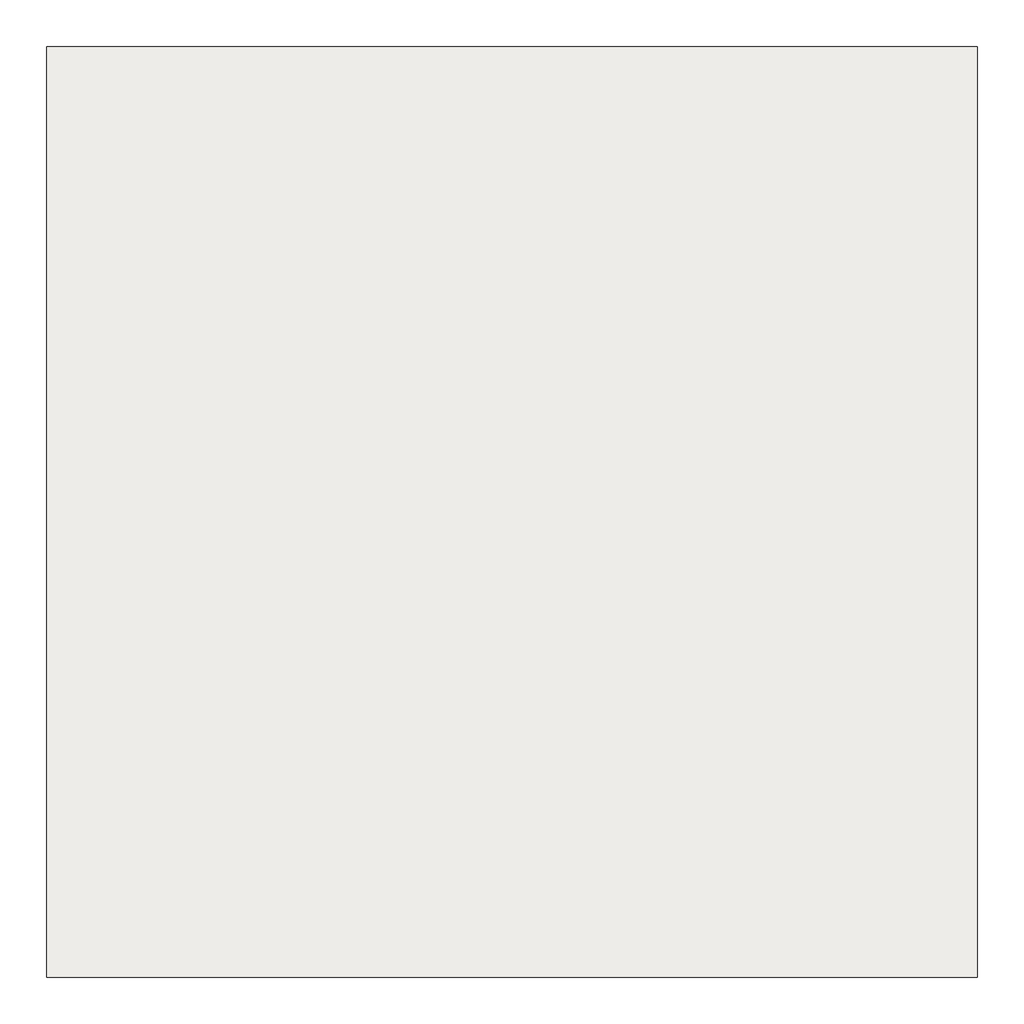
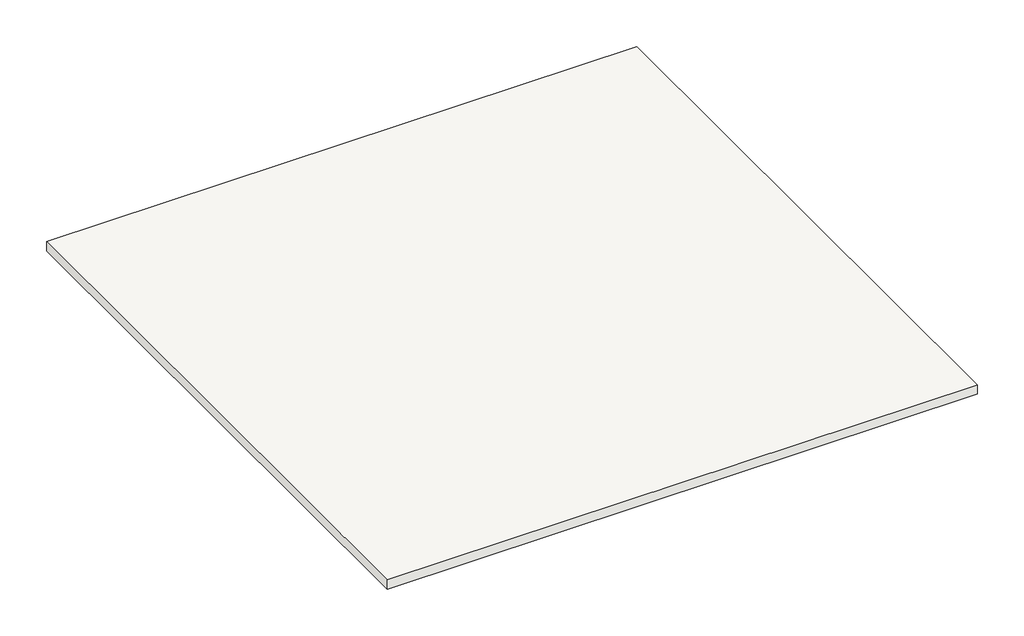
# One storey: 1 slab.
"""IFC4 building model written with IfcOpenShell, lengths in millimetres."""

from ifc_helpers import new_model, si_unit, frame, origin, place, context, project, spatial, polyline, outline, extrude, element, save

model = new_model("IFC4")

# Units and contexts
model_context = context("Model", 3, world=origin())
ifc_project = project(units=[si_unit("LENGTHUNIT", "METRE", prefix="MILLI")], contexts=[model_context])

# Site, building, storey
site = spatial("IfcSite", under=ifc_project)
building = spatial("IfcBuilding", under=site)
storey = spatial("IfcBuildingStorey", under=building, Elevation=9144.0)

# Slab
placement = place(None, origin())
element("IfcSlab", 1, ObjectType="6\" Foundation Slab", at=placement, inside=storey, context=model_context, shape_type="SweptSolid", body=[
    extrude(outline(polyline([(-12698.1609662, 12623.5972109), (-12698.1609662, 3479.5972109), (-21842.1609662, 3479.5972109), (-21842.1609662, 12623.5972109), (-12698.1609662, 12623.5972109)])), frame((0.0, 0.0, 8991.6), z_axis=(0.0, 0.0, 1.0), x_axis=(1.0, 0.0, 0.0)), (0.0, 0.0, 1.0), 152.4),
])

save(model, "model.ifc")

# Revit data of these elements
# Type "6\" Foundation Slab"
#   Layers, outside or top first: 0' - 6" "Concrete, Cast-in-Place gray" (function 1)
# Element 1 (IfcSlab, "6\" Foundation Slab")
#   Height Offset From Level = 0' - 0"
#   built-in parameter 1001954 = 1
#   Phase Created = New Construction
#   Materials on its faces: "Concrete, Cast-in-Place gray"
# Materials
#   "Concrete, Cast-in-Place gray": class "Concrete", colour RGB 192 192 192, transparency 0, Description = "Cast-in-place concrete", Cost = 0
